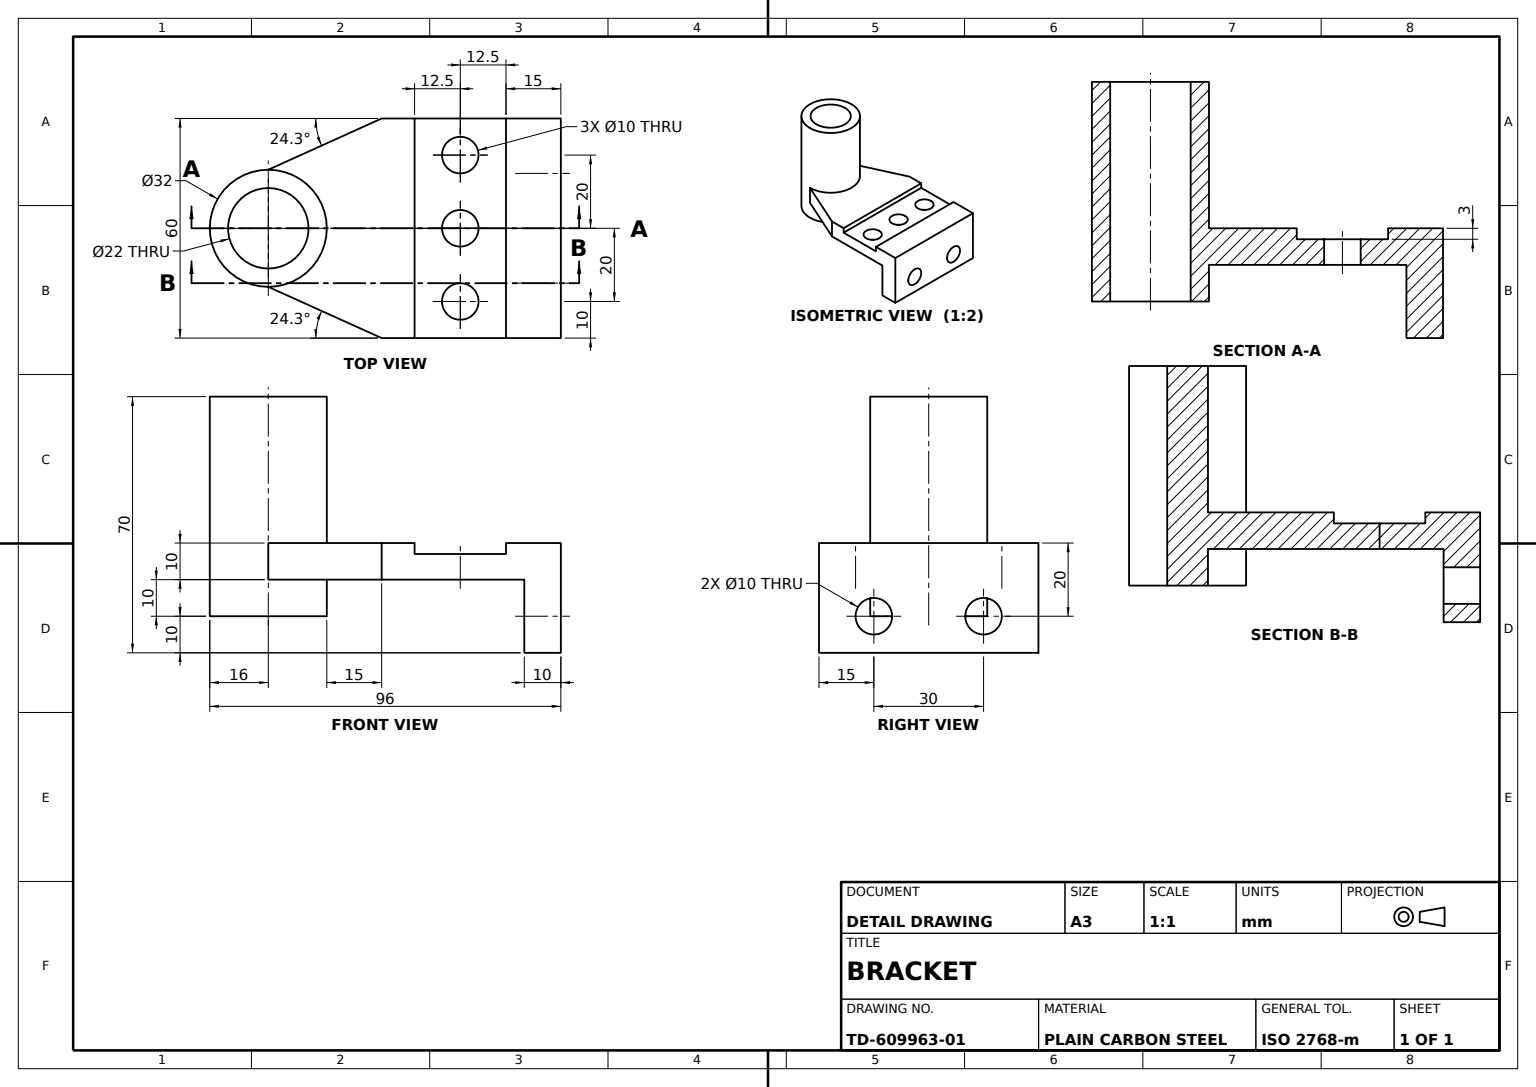
SolidWorks part; units mm, degrees
material "Plain Carbon Steel"
ref_plane "Front Plane" through (0, 0, 0) normal (0, 0, 1) x (1, 0, 0)
ref_plane "Top Plane" through (0, 0, 0) normal (0, 1, 0) x (1, 0, 0)
ref_plane "Right Plane" through (0, 0, 0) normal (1, 0, 0) x (0, 0, -1)
sketch "Bracket Profile Sketch" plane through (0, 0, 0) normal (0, 0, 1) x (1, 0, 0)
  line L0 (0, 0) -> (70, 0)
  line L1 (70, 0) -> (70, -20)
  line L2 (70, -20) -> (80, -20)
  line L3 (80, -20) -> (80, 10)
  line L7 (0, 10) -> (0, 0)
  line L8 (0, 10) -> (40, 10)
  line L9 (40, 10) -> (40, 7)
  line L10 (40, 7) -> (65, 7)
  line L11 (65, 7) -> (65, 10)
  line L12 (65, 10) -> (80, 10)
  dimension "D1" = 30
  dimension "D2" = 40
  dimension "D3" = 70
  dimension "D4" = 10
  dimension "D5" = 10
  dimension "D6" = 15
  dimension "D7" = 3
extrude "Bracket Body 60mm" add sketch "Bracket Profile Sketch" along normal mid plane 60
sketch "Top Holes Sketch" plane through (80, 0, 0) normal (1, 0, 0) x (0, 0, -1)
  line L0 (30, -20) -> (30, -10) construction
  line L1 (30, -20) -> (30, 10) construction
  line L2 (30, -10) -> (15, -10) construction
  line L3 (15, -10) -> (-15, -10) construction
  line L4 (0, 0) -> (0, -10) construction
  circle A0 centre (-15, -10) radius 5
  circle A1 centre (15, -10) radius 5
  dimension "D3" = 10
  dimension "D4" = 10
  dimension "D1" = 15
  dimension "D2" = 30
  dimension "D5" = 15
  dimension "D6" = 18.0278
extrude "Top Holes" cut sketch "Top Holes Sketch" against normal blind 15
sketch "Top Groove Sketch" plane through (0, 10, 0) normal (0, 1, 0) x (1, 0, 0)
  line L1 (40, 30) -> (0, 30) construction
  line L2 (31, 30) -> (0, 16)
  line L3 (0, -30) -> (0, 30) construction
  line L4 (0, -16) -> (0, 16)
  line L5 (0, 0) -> (40, 0) construction
  line L6 (40, -30) -> (40, 30) construction
  line L8 (31, -30) -> (0, -16)
  line L9 (31, 30) -> (0, 30)
  line L10 (0, 30) -> (0, 16)
  line L11 (0, -16) -> (0, -30)
  line L12 (0, -30) -> (31, -30)
  line M5 (40, 30) -> (0, 30)
  line M6 (0, 30) -> (0, -30)
  line M7 (0, -30) -> (40, -30)
  dimension "D1" = 34.0147
  dimension "D2" = 32
extrude "Top Groove Cut" cut sketch "Top Groove Sketch" against normal blind 15 contours L2 M5 M6 | L8 M7 M6
sketch "Hinge Tube Upper Sketch" plane through (0, 10, 0) normal (0, 1, 0) x (1, 0, 0)
  circle A0 centre (0, 0) radius 16
  circle A1 centre (0, 0) radius 11
  dimension "D1" = 32
  dimension "D2" = 22
extrude "Hinge Tube Upper Ø32x40" add sketch "Hinge Tube Upper Sketch" along normal blind 40
sketch "Hinge Tube Lower Sketch" plane through (0, 10, 0) normal (0, 1, 0) x (1, 0, 0)
  circle A0 centre (0, 0) radius 16
  circle A1 centre (0, 0) radius 11
  dimension "D1" = 32
  dimension "D2" = 22
extrude "Hinge Tube Lower Ø32x20" add sketch "Hinge Tube Lower Sketch" against normal blind 20
sketch "Hinge Bore Sketch" plane through (0, 10, 0) normal (0, 1, 0) x (1, 0, 0)
  circle A0 centre (0, 0) radius 11
  dimension "D1" = 22
extrude "Hinge Bore Ø22" cut sketch "Hinge Bore Sketch" against normal blind 20
sketch "Side Holes Sketch" plane through (0, 7, 0) normal (0, 1, 0) x (1, 0, 0)
  line L0 (40, -30) -> (40, -20) construction
  line L1 (40, -30) -> (40, 30) construction
  line L2 (40, -20) -> (52.5, -20) construction
  line L3 (40, 0) -> (65, 0) construction
  line L4 (65, -30) -> (65, 30) construction
  circle A0 centre (52.5, -20) radius 5
  circle A1 centre (52.5, 0) radius 5
  circle A2 centre (52.5, 20) radius 5
  dimension "D1" = 10
  dimension "D2" = 10
  dimension "D3" = 10
  dimension "D4" = 20
extrude "Side Holes" cut sketch "Side Holes Sketch" against normal blind 20
